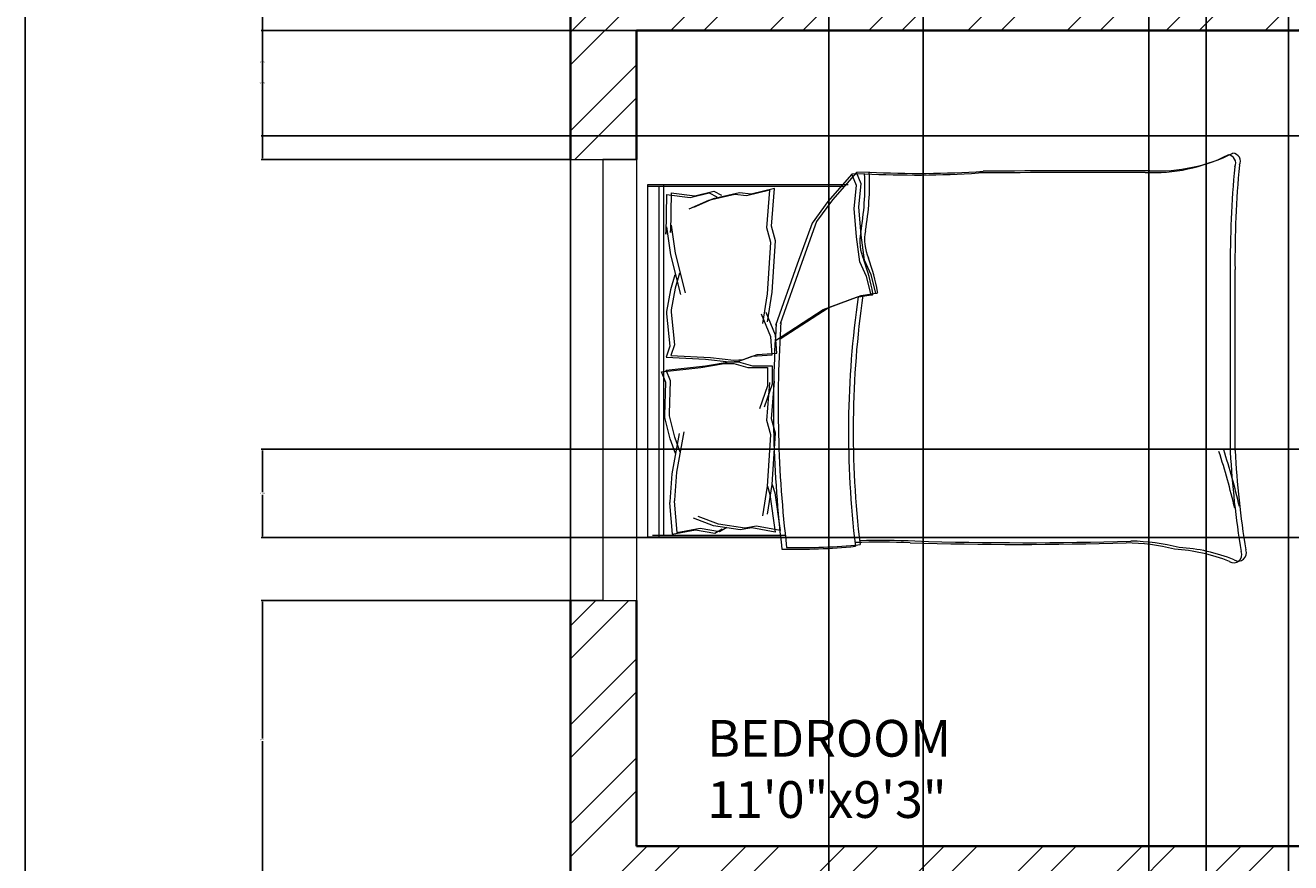
# Model space of a CAD drawing. Units: inches. Extents: x 1748 to 2382, y 1346 to 2284.
# Tile 8 of 26: x 1748 to 1920, y 1857 to 1971. Entities that reach past the tile are written whole.
import ezdxf

# ---------------------------------------------------------------- set-up
doc = ezdxf.new("R2010")
doc.units = ezdxf.units.IN
for name, color, linetype, lineweight in [('A-ANNO-DIMS', 2, 'Continuous', 18), ('A-ANNO-TTLB', 7, 'Continuous', 25), ('A-AREA-IDEN', 7, 'Continuous', 18), ('A-FURN', 8, 'Continuous', 13), ('A-GLAZ', 191, 'Continuous', 18), ('A-WALL', 7, 'Continuous', 35), ('A-WALL-PATT', 9, 'Continuous', 13)]:
    doc.layers.add(name, color=color, linetype=linetype, lineweight=lineweight)
doc.styles.get("Standard").update_dxf_attribs({"font": 'arial.ttf'})
doc.dimstyles.get("Standard").update_dxf_attribs({"dimtxt": 0.18, "dimasz": 0.18, "dimexe": 0.18, "dimexo": 0.0625, "dimgap": 0.09, "dimtad": 0, "dimtih": 1, "dimtoh": 1, "dimdec": 4, "dimzin": 0, "dimdsep": 46, "dimtxsty": 'Standard', "dimcen": 0.09, "dimadec": 0, "dimazin": 0, "dimtfac": 1, "dimtdec": 4, "dimtofl": 0, "dimtmove": 0, "dimatfit": 3, "dimfxl": 1, "dimtolj": 1, "dimtzin": 0, "dimarcsym": 0})

# ---------------------------------------------------------------- blocks, each defined once
blk = doc.blocks.new('BED-DOUBLE')
for p, q in [((3.48, 63.33), (3.48, 81.44)), ((3.48, 63.33), (3.48, 81.44)), ((3.48, 81.44), (51.49, 81.44)), ((51.27, 81.44), (51.27, 54.83)), ((51.27, 81.44), (51.27, 54.83)), ((51.49, 81.44), (51.49, 80.8)), ((3.48, 79.91), (51.27, 79.91)), ((3.48, 79.91), (51.27, 79.91)), ((3.7, 62.69), (3.7, 80.8)), ((3.7, 62.69), (3.7, 80.8)), ((3.7, 79.27), (51.49, 79.27)), ((3.7, 79.27), (51.49, 79.27)), ((24.54, 78.99), (25.98, 79.57)), ((24.54, 78.99), (25.98, 79.57)), ((25.98, 79.57), (26.56, 74.22)), ((25.98, 79.57), (26.56, 74.22)), ((51.49, 80.8), (51.49, 54.19)), ((51.49, 80.8), (51.49, 54.19)), ((3.89, 78.13), (4.47, 74.95)), ((3.9, 78.11), (8.18, 78.43)), ((3.9, 78.11), (8.18, 78.43)), ((3.9, 78.13), (4.47, 74.95)), ((4.12, 77.49), (4.7, 74.31)), ((4.12, 77.49), (4.7, 74.31)), ((4.13, 77.47), (8.41, 77.8)), ((4.13, 77.47), (8.41, 77.8)), ((8.18, 78.43), (8.29, 78.42)), ((8.18, 78.43), (8.28, 78.42)), ((8.28, 78.42), (12.11, 78.13)), ((8.29, 78.42), (12.11, 78.13)), ((8.41, 77.8), (8.51, 77.78)), ((8.41, 77.8), (8.51, 77.78)), ((8.51, 77.78), (12.34, 77.49)), ((8.51, 77.78), (12.34, 77.49)), ((12.11, 78.13), (17.6, 77.12)), ((12.11, 78.13), (17.6, 77.12)), ((12.34, 77.49), (17.83, 76.48)), ((12.34, 77.49), (17.83, 76.48)), ((14.86, 77.69), (16.88, 78.42)), ((14.86, 77.69), (16.88, 78.42)), ((15.08, 77.05), (17.11, 77.78)), ((15.08, 77.05), (17.11, 77.78)), ((16.88, 78.42), (19.77, 79.14)), ((16.88, 78.42), (19.77, 79.14)), ((17.11, 77.78), (20, 78.5)), ((17.11, 77.78), (20, 78.5)), ((19.77, 79.14), (20.09, 79.14)), ((19.77, 79.14), (20.09, 79.14)), ((20, 78.5), (20.32, 78.5)), ((20, 78.5), (20.32, 78.5)), ((20.09, 79.14), (24.54, 78.99)), ((20.09, 79.14), (24.54, 78.99)), ((20.32, 78.5), (24.77, 78.36)), ((20.32, 78.5), (24.77, 78.36)), ((24.77, 78.36), (26.21, 78.93)), ((24.77, 78.36), (26.21, 78.93)), ((26.21, 78.93), (26.79, 73.58)), ((26.21, 78.93), (26.79, 73.58)), ((27.98, 78.95), (27.73, 73.58)), ((27.98, 78.95), (27.73, 73.58)), ((28.21, 78.31), (27.96, 72.94)), ((28.21, 78.31), (27.96, 72.94)), ((29.46, 78.46), (27.98, 78.95)), ((29.46, 78.46), (27.98, 78.95)), ((29.68, 77.83), (28.21, 78.31)), ((29.68, 77.83), (28.21, 78.31)), ((33.88, 78.89), (29.46, 78.46)), ((33.88, 78.89), (29.46, 78.46)), ((34.11, 78.25), (29.68, 77.83)), ((34.11, 78.25), (29.68, 77.83)), ((34.21, 78.91), (33.88, 78.89)), ((34.2, 78.91), (33.88, 78.89)), ((34.43, 78.27), (34.11, 78.25)), ((34.43, 78.27), (34.11, 78.25)), ((37.14, 78.37), (34.2, 78.91)), ((37.14, 78.37), (34.21, 78.91)), ((37.36, 77.73), (34.43, 78.27)), ((37.36, 77.73), (34.43, 78.27)), ((41.91, 78.37), (36.5, 77.02)), ((41.91, 78.37), (36.5, 77.02)), ((42.14, 77.73), (36.72, 76.38)), ((42.14, 77.73), (36.72, 76.38)), ((39.2, 77.77), (37.14, 78.37)), ((39.2, 77.77), (37.14, 78.37)), ((39.43, 77.13), (37.36, 77.73)), ((39.43, 77.13), (37.36, 77.73)), ((45.71, 78.9), (41.91, 78.37)), ((45.71, 78.9), (41.91, 78.37)), ((45.94, 78.26), (42.14, 77.73)), ((45.94, 78.26), (42.14, 77.73)), ((50.11, 78.89), (44.71, 78.98)), ((44.71, 78.98), (45.71, 78.9)), ((50.11, 78.89), (44.71, 78.98)), ((44.71, 78.98), (45.71, 78.9)), ((50.34, 78.25), (44.94, 78.34)), ((44.94, 78.34), (45.94, 78.26)), ((50.34, 78.25), (44.94, 78.34)), ((44.94, 78.34), (45.94, 78.26)), ((50.11, 78.89), (49.73, 75.68)), ((50.11, 78.89), (49.73, 75.68)), ((50.34, 78.25), (49.96, 75.04)), ((50.34, 78.25), (49.96, 75.04)), ((49.31, 73.19), (48.13, 75.87)), ((49.31, 73.19), (48.13, 75.87)), ((4.47, 74.95), (4.04, 72.34)), ((4.47, 74.95), (4.04, 72.34)), ((4.7, 74.31), (4.27, 71.7)), ((4.7, 74.31), (4.27, 71.7)), ((5.05, 72.49), (6.06, 75.24)), ((5.05, 72.49), (6.06, 75.24)), ((5.28, 71.85), (6.29, 74.6)), ((5.28, 71.85), (6.29, 74.6)), ((26.56, 74.22), (27.14, 71.04)), ((26.56, 74.22), (27.14, 71.04)), ((49.54, 72.55), (48.36, 75.23)), ((49.54, 72.55), (48.36, 75.23)), ((49.73, 75.68), (50.33, 73.11)), ((49.73, 75.68), (50.33, 73.11)), ((49.96, 75.04), (50.56, 72.47)), ((49.96, 75.04), (50.56, 72.47)), ((4.04, 72.34), (4.62, 71.33)), ((4.04, 72.34), (4.62, 71.33)), ((4.47, 68.87), (5.05, 72.49)), ((4.47, 68.87), (5.05, 72.49)), ((26.79, 73.58), (27.37, 70.4)), ((26.79, 73.58), (27.37, 70.4)), ((27.73, 73.58), (27.35, 70.37)), ((27.73, 73.58), (27.36, 70.37)), ((27.96, 72.94), (27.58, 69.73)), ((27.96, 72.94), (27.58, 69.73)), ((50.11, 69.61), (49.31, 73.19)), ((50.11, 69.61), (49.31, 73.19)), ((50.34, 68.98), (49.54, 72.55)), ((50.34, 68.98), (49.54, 72.55)), ((50.33, 73.11), (49.81, 72.06)), ((50.33, 73.11), (49.81, 72.06)), ((50.56, 72.47), (50.04, 71.42)), ((50.56, 72.47), (50.04, 71.42)), ((4.27, 71.7), (4.85, 70.69)), ((4.27, 71.7), (4.85, 70.69)), ((4.7, 68.23), (5.28, 71.85)), ((4.7, 68.23), (5.28, 71.85)), ((27.14, 71.04), (27.14, 69.74)), ((27.14, 71.04), (27.14, 69.74)), ((4.76, 67.28), (4.47, 68.87)), ((4.76, 67.28), (4.47, 68.87)), ((27.14, 69.74), (26.56, 67.86)), ((27.14, 69.74), (26.56, 67.86)), ((27.37, 69.1), (26.79, 67.22)), ((27.37, 69.1), (26.79, 67.22)), ((27.35, 70.37), (27.44, 69.07)), ((27.36, 70.37), (27.44, 69.07)), ((27.37, 70.4), (27.37, 69.1)), ((27.37, 70.4), (27.37, 69.1)), ((27.44, 69.07), (28.13, 67.23)), ((27.44, 69.07), (28.13, 67.23)), ((27.58, 69.73), (27.66, 68.43)), ((27.58, 69.73), (27.66, 68.43)), ((49.92, 68.01), (50.11, 69.61)), ((49.92, 68.01), (50.11, 69.61)), ((50.15, 67.37), (50.34, 68.98)), ((50.15, 67.37), (50.34, 68.98)), ((4.18, 64.1), (4.76, 67.28)), ((4.18, 64.1), (4.76, 67.28)), ((4.99, 66.64), (4.7, 68.23)), ((4.99, 66.64), (4.7, 68.23)), ((26.56, 67.86), (26.56, 65.18)), ((26.56, 67.86), (26.56, 65.18)), ((26.79, 67.22), (26.79, 64.54)), ((26.79, 67.22), (26.79, 64.54)), ((27.66, 68.43), (28.36, 66.59)), ((27.66, 68.43), (28.36, 66.59)), ((28.13, 67.23), (28.3, 64.55)), ((28.13, 67.23), (28.3, 64.55)), ((50.7, 64.87), (49.92, 68.01)), ((50.7, 64.87), (49.92, 68.01)), ((50.93, 64.23), (50.15, 67.37)), ((50.93, 64.23), (50.15, 67.37)), ((4.41, 63.46), (4.99, 66.64)), ((4.41, 63.46), (4.99, 66.64)), ((6.38, 65.81), (10.41, 65.15)), ((6.38, 65.81), (10.41, 65.15)), ((24.1, 65.18), (20.96, 66.27)), ((24.1, 65.18), (20.96, 66.27)), ((24.33, 64.54), (21.19, 65.63)), ((24.33, 64.54), (21.19, 65.63)), ((28.36, 66.59), (28.53, 63.91)), ((28.36, 66.59), (28.53, 63.91)), ((30.75, 64.7), (33.82, 65.99)), ((30.75, 64.7), (33.82, 65.99)), ((32.56, 65.81), (36.6, 65.15)), ((32.56, 65.81), (36.6, 65.15)), ((9.28, 64.83), (4.18, 64.1)), ((9.28, 64.83), (4.18, 64.1)), ((9.51, 64.19), (4.41, 63.46)), ((9.51, 64.19), (4.41, 63.46)), ((6.61, 65.18), (10.64, 64.51)), ((6.61, 65.18), (10.64, 64.51)), ((10.41, 65.15), (9.28, 64.83)), ((10.41, 65.15), (9.28, 64.83)), ((10.64, 64.51), (9.51, 64.19)), ((10.64, 64.51), (9.51, 64.19)), ((10.41, 65.15), (17.42, 64.72)), ((10.41, 65.15), (17.42, 64.72)), ((10.64, 64.51), (17.65, 64.08)), ((10.64, 64.51), (17.65, 64.08)), ((17.42, 64.72), (19.38, 65.27)), ((17.42, 64.72), (19.38, 65.27)), ((17.65, 64.08), (19.61, 64.64)), ((17.65, 64.08), (19.61, 64.64)), ((19.38, 65.27), (24.52, 64.87)), ((19.38, 65.27), (24.52, 64.87)), ((19.61, 64.64), (24.74, 64.23)), ((19.61, 64.64), (24.74, 64.23)), ((26.56, 65.18), (24.1, 65.18)), ((26.56, 65.18), (24.1, 65.18)), ((26.79, 64.54), (24.33, 64.54)), ((26.79, 64.54), (24.33, 64.54)), ((28.3, 64.55), (30.75, 64.7)), ((28.3, 64.55), (30.75, 64.7)), ((28.53, 63.91), (30.98, 64.06)), ((28.53, 63.91), (30.98, 64.06)), ((30.26, 64.06), (34.45, 57.57)), ((30.26, 64.06), (34.45, 57.57)), ((30.98, 64.06), (34.05, 65.35)), ((30.98, 64.06), (34.05, 65.35)), ((40.64, 61.13), (32.31, 64.06)), ((40.64, 61.13), (32.31, 64.06)), ((32.79, 65.18), (36.83, 64.51)), ((32.79, 65.18), (36.82, 64.51)), ((36.6, 65.15), (43.61, 64.72)), ((36.6, 65.15), (43.61, 64.72)), ((36.82, 64.51), (43.83, 64.08)), ((36.83, 64.51), (43.83, 64.08)), ((43.61, 64.72), (45.57, 65.27)), ((43.61, 64.72), (45.57, 65.27)), ((43.83, 64.08), (45.8, 64.64)), ((43.83, 64.08), (45.79, 64.64)), ((45.57, 65.27), (50.7, 64.87)), ((45.57, 65.27), (50.7, 64.87)), ((45.79, 64.64), (50.93, 64.23)), ((45.8, 64.64), (50.93, 64.23)), ((30.49, 63.42), (34.68, 56.93)), ((30.49, 63.42), (34.68, 56.93)), ((40.87, 60.49), (32.53, 63.42)), ((40.87, 60.49), (32.53, 63.42)), ((46.22, 59.11), (40.64, 61.13)), ((46.22, 59.11), (40.64, 61.13)), ((46.45, 58.48), (40.87, 60.49)), ((46.45, 58.48), (40.87, 60.49)), ((49.16, 56.95), (46.22, 59.11)), ((49.16, 56.95), (46.22, 59.11)), ((34.45, 57.57), (36.15, 53.08)), ((34.45, 57.57), (36.15, 53.08)), ((34.68, 56.93), (36.38, 52.44)), ((34.68, 56.93), (36.38, 52.44)), ((49.39, 56.31), (46.45, 58.48)), ((49.39, 56.31), (46.45, 58.48)), ((52.87, 53.7), (49.16, 56.95)), ((52.87, 53.7), (49.16, 56.95)), ((53.1, 53.06), (49.39, 56.31)), ((53.1, 53.06), (49.39, 56.31)), ((44.36, 53.08), (48.23, 53.39)), ((44.36, 53.08), (48.23, 53.39)), ((48.23, 53.39), (51.33, 53.08)), ((48.23, 53.39), (51.33, 53.08)), ((51.33, 53.08), (52.87, 53.7)), ((51.33, 53.08), (52.87, 53.7)), ((52.95, 51.95), (52.87, 53.7, 3.87)), ((52.95, 51.95), (52.87, 53.7, 3.87)), ((36.15, 53.08), (36.46, 51.07)), ((36.15, 53.08), (36.46, 51.07)), ((36.38, 52.44), (36.69, 50.43)), ((36.38, 52.44), (36.69, 50.43)), ((36.46, 51.07), (38.94, 51.69)), ((36.46, 51.07), (38.94, 51.69)), ((38.94, 51.69), (40.95, 52.61)), ((38.94, 51.69), (40.95, 52.61)), ((39.17, 51.05), (41.18, 51.97)), ((39.17, 51.05), (41.18, 51.97)), ((40.95, 52.61), (44.36, 53.08)), ((40.95, 52.61), (44.36, 53.08)), ((41.18, 51.97), (44.59, 52.44)), ((41.18, 51.97), (44.59, 52.44)), ((44.59, 52.44), (48.46, 52.75)), ((44.59, 52.44), (48.46, 52.75)), ((48.46, 52.75), (51.56, 52.44)), ((48.46, 52.75), (51.56, 52.44)), ((51.56, 52.44), (53.1, 53.06)), ((51.56, 52.44), (53.1, 53.06)), ((53.18, 51.31), (53.1, 53.06, 3.87)), ((53.18, 51.31), (53.1, 53.06, 3.87)), ((36.69, 50.43), (39.17, 51.05)), ((36.69, 50.43), (39.17, 51.05)), ((15.06, 2.2), (39.68, 2.2)), ((15.06, 2.2), (39.68, 2.2)), ((15.29, 1.56), (39.91, 1.56)), ((15.29, 1.56), (39.91, 1.56))]:
    blk.add_line(p, q)
for centre, radius, start, end in [((21.36, -100.61), 164.97, 86.0865, 96.7821), ((21.36, -100.61), 164.97, 86.0865, 96.7821), ((21.59, -101.25), 164.97, 86.0865, 96.7821), ((21.59, -101.25), 164.97, 86.0865, 96.7821), ((85.16, 61.35), 83.31, 178.7218, 185.604), ((85.16, 61.35), 83.31, 178.7218, 185.604), ((85.39, 60.71), 83.31, 178.7218, 185.604), ((85.39, 60.71), 83.31, 178.7218, 185.604), ((17.76, -74.87), 129.02, 81.7845, 96.9006), ((17.76, -74.87), 129.02, 81.7845, 96.9006), ((17.98, -75.51), 129.02, 81.7845, 96.9006), ((17.98, -75.51), 129.02, 81.7845, 96.9006), ((-167.31, 50.27), 170.11, 358.4762, 1.0082), ((-167.31, 50.27), 170.11, 358.4762, 1.0082), ((-167.08, 49.63), 170.11, 358.4762, 1.0082), ((-167.08, 49.63), 170.11, 358.4762, 1.0082), ((31.15, 79.96), 29.65, 280.6617, 289.8806), ((31.15, 79.96), 29.65, 280.6617, 289.8806), ((43.74, 46.38), 6.22, 78.6608, 113.7384), ((43.74, 46.38), 6.22, 78.6608, 113.7384), ((43.97, 45.74), 6.22, 78.6608, 113.7384), ((43.97, 45.74), 6.22, 78.6608, 113.7384), ((51.33, 88.1), 36.18, 259.8763, 272.5657), ((51.33, 88.1), 36.18, 259.8763, 272.5657), ((51.56, 87.46), 36.18, 259.8763, 272.5657), ((51.56, 87.46), 36.18, 259.8763, 272.5657), ((182.27, 45.13), 129.5, 176.9791, 183.8365), ((182.27, 45.13), 129.5, 176.9791, 183.8365), ((36.64, 51), 0.185, 160.2464, 271.1377), ((36.64, 51), 0.185, 160.2464, 271.1377), ((36.87, 50.36), 0.185, 160.2464, 271.1377), ((36.86, 50.36), 0.185, 160.2464, 271.1377), ((31.38, 79.32), 29.65, 280.6617, 289.8806), ((31.38, 79.32), 29.65, 280.6617, 289.8806), ((182.49, 44.49), 129.5, 176.9791, 183.8365), ((182.49, 44.49), 129.5, 176.9791, 183.8365), ((484.82, 30.83), 482.31, 178.2277, 181.7185), ((484.82, 30.83), 482.31, 178.2277, 181.7185), ((485.05, 30.19), 482.31, 178.2277, 181.7185), ((485.05, 30.19), 482.31, 178.2277, 181.7185), ((-4508.74, 13.62), 4561.86, 0.00217, 0.28689), ((-4508.74, 13.62), 4561.86, 0.00217, 0.28689), ((-4508.51, 12.98), 4561.86, 0.00217, 0.28689), ((-4508.51, 12.98), 4561.86, 0.00217, 0.28689), ((-26.9, 16.93), 29.63, 346.0648, 358.9113), ((-26.9, 16.93), 29.63, 346.0648, 358.9113), ((-26.67, 16.29), 29.63, 346.0648, 358.9113), ((-26.67, 16.29), 29.63, 346.0648, 358.9113), ((76.16, 12.78), 23.07, 177.4714, 206.4681), ((76.16, 12.78), 23.07, 177.4714, 206.4681), ((76.39, 12.14), 23.07, 177.4714, 206.4681), ((76.39, 12.14), 23.07, 177.4714, 206.4681), ((-21.66, 11.17), 23.56, 337.9751, 356.652), ((-21.66, 11.17), 23.56, 337.9751, 356.652), ((-21.43, 10.53), 23.56, 337.9751, 356.652), ((-21.43, 10.53), 23.56, 337.9751, 356.652), ((-17.22, 105.16), 106.46, 283.3832, 287.7053), ((-17.22, 105.16), 106.46, 283.3832, 287.7053), ((1.09, 1.73), 1.09, 146.1736, 293.4781), ((1.09, 1.73), 1.09, 146.1736, 293.4781), ((21.43, -119.39), 121.76, 92.9958, 99.4091), ((21.43, -119.39), 121.76, 92.9958, 99.4091), ((-16.99, 104.52), 106.46, 283.3832, 287.7053), ((-16.99, 104.52), 106.46, 283.3832, 287.7053), ((41.15, -130.83), 133.04, 84.4998, 90.6351), ((41.15, -130.83), 133.04, 84.4998, 90.6351), ((54.41, 2.57), 1.1, 242.6588, 356.02), ((54.41, 2.57), 1.1, 242.6588, 356.02), ((54.64, 1.93), 1.1, 242.6588, 356.02), ((54.64, 1.93), 1.1, 242.6588, 356.02), ((1.32, 1.09), 1.09, 146.1736, 293.4781), ((1.32, 1.09), 1.09, 146.1736, 293.4781), ((21.66, -120.03), 121.76, 92.9958, 99.4091), ((21.66, -120.03), 121.76, 92.9958, 99.4091), ((41.38, -131.47), 133.04, 84.4998, 90.6351), ((41.38, -131.47), 133.04, 84.4998, 90.6351)]:
    blk.add_arc(centre, radius, start, end)
blk = doc.blocks.new('*D37')
at = {"layer": 'A-ANNO-DIMS', "color": 0, "lineweight": -2, "transparency": 16777216}
for p, q in [((2031.9, 1970.35), (1779.88, 1970.35)), ((1780.06, 1970.17), (1780.06, 1963.37)), ((1780.06, 1956.2), (1780.06, 1963.01)), ((2031.9, 1956.02), (1779.88, 1956.02))]:
    blk.add_line(p, q, dxfattribs=at)
at = {"layer": 'A-ANNO-DIMS', "color": 0, "transparency": 16777216}
for points in [[(1780.03, 1970.17), (1780.09, 1970.17), (1780.06, 1970.35)], [(1780.03, 1956.2), (1780.09, 1956.2), (1780.06, 1956.02)]]:
    blk.add_solid(points, dxfattribs=at)
at = {"layer": 'Defpoints', "color": 0, "transparency": 16777216}
for p in [(1780.06, 1970.35), (2031.96, 1970.35), (2031.96, 1956.02)]:
    blk.add_point(p, dxfattribs=at)
at = {"layer": 'A-ANNO-DIMS', "color": 0, "transparency": 16777216, "insert": (1780.06, 1963.19), "char_height": 0.18, "attachment_point": 5}
blk.add_mtext('\\A1;14.325', dxfattribs=at)
blk = doc.blocks.new('*D41')
at = {"layer": 'A-ANNO-DIMS', "color": 0, "lineweight": -2, "transparency": 16777216}
for p, q in [((1821.96, 1854.91), (1821.96, 2274.93)), ((1822.14, 2274.75), (1839.16, 2274.75)), ((1856.96, 2274.75), (1839.95, 2274.75)), ((1857.14, 1854.91), (1857.14, 2274.93))]:
    blk.add_line(p, q, dxfattribs=at)
at = {"layer": 'A-ANNO-DIMS', "color": 0, "transparency": 16777216}
for points in [[(1822.14, 2274.78), (1822.14, 2274.72), (1821.96, 2274.75)], [(1856.96, 2274.78), (1856.96, 2274.72), (1857.14, 2274.75)]]:
    blk.add_solid(points, dxfattribs=at)
at = {"layer": 'Defpoints', "color": 0, "transparency": 16777216}
for p in [(1857.14, 2274.75), (1821.96, 1854.85), (1857.14, 1854.85)]:
    blk.add_point(p, dxfattribs=at)
at = {"layer": 'A-ANNO-DIMS', "color": 0, "transparency": 16777216, "insert": (1839.55, 2274.75), "char_height": 0.18, "attachment_point": 5}
blk.add_mtext('\\A1;35.18', dxfattribs=at)
blk = doc.blocks.new('*D44')
at = {"layer": 'A-ANNO-DIMS', "color": 0, "lineweight": -2, "transparency": 16777216}
for p, q in [((1821.9, 1892.79), (1779.88, 1892.79)), ((1780.06, 1892.61), (1780.06, 1874)), ((1780.06, 1855.03), (1780.06, 1873.64)), ((1821.9, 1854.85), (1779.88, 1854.85))]:
    blk.add_line(p, q, dxfattribs=at)
at = {"layer": 'A-ANNO-DIMS', "color": 0, "transparency": 16777216}
for points in [[(1780.03, 1892.61), (1780.09, 1892.61), (1780.06, 1892.79)], [(1780.03, 1855.03), (1780.09, 1855.03), (1780.06, 1854.85)]]:
    blk.add_solid(points, dxfattribs=at)
at = {"layer": 'Defpoints', "color": 0, "transparency": 16777216}
for p in [(1780.06, 1892.79), (1821.96, 1892.79), (1821.96, 1854.85)]:
    blk.add_point(p, dxfattribs=at)
at = {"layer": 'A-ANNO-DIMS', "color": 0, "transparency": 16777216, "insert": (1780.06, 1873.82), "char_height": 0.18, "attachment_point": 5}
blk.add_mtext('\\A1;37.94', dxfattribs=at)
blk = doc.blocks.new('*D50')
at = {"layer": 'A-ANNO-DIMS', "color": 0, "lineweight": -2, "transparency": 16777216}
for p, q in [((1869.96, 2223.79), (1869.96, 1360.47)), ((1908.44, 2223.79), (1908.44, 1360.47)), ((1870.14, 1360.65), (1888.81, 1360.65)), ((1908.26, 1360.65), (1889.6, 1360.65))]:
    blk.add_line(p, q, dxfattribs=at)
at = {"layer": 'A-ANNO-DIMS', "color": 0, "transparency": 16777216}
for points in [[(1870.14, 1360.68), (1870.14, 1360.62), (1869.96, 1360.65)], [(1908.26, 1360.68), (1908.26, 1360.62), (1908.44, 1360.65)]]:
    blk.add_solid(points, dxfattribs=at)
at = {"layer": 'Defpoints', "color": 0, "transparency": 16777216}
for p in [(1869.96, 2223.85), (1908.44, 2223.85), (1908.44, 1360.65)]:
    blk.add_point(p, dxfattribs=at)
at = {"layer": 'A-ANNO-DIMS', "color": 0, "transparency": 16777216, "insert": (1889.2, 1360.65), "char_height": 0.18, "attachment_point": 5}
blk.add_mtext('\\A1;38.48', dxfattribs=at)
blk = doc.blocks.new('*D56')
at = {"layer": 'A-ANNO-DIMS', "color": 0, "lineweight": -2, "transparency": 16777216}
for p, q in [((2288.4, 1913.35), (1779.88, 1913.35)), ((1780.06, 1913.17), (1780.06, 1907.52)), ((1780.06, 1901.51), (1780.06, 1907.16)), ((2288.4, 1901.33), (1779.88, 1901.33))]:
    blk.add_line(p, q, dxfattribs=at)
at = {"layer": 'A-ANNO-DIMS', "color": 0, "transparency": 16777216}
for points in [[(1780.03, 1913.17), (1780.09, 1913.17), (1780.06, 1913.35)], [(1780.03, 1901.51), (1780.09, 1901.51), (1780.06, 1901.33)]]:
    blk.add_solid(points, dxfattribs=at)
at = {"layer": 'Defpoints', "color": 0, "transparency": 16777216}
for p in [(1780.06, 1913.35), (2288.46, 1913.35), (2288.46, 1901.33)]:
    blk.add_point(p, dxfattribs=at)
at = {"layer": 'A-ANNO-DIMS', "color": 0, "transparency": 16777216, "insert": (1780.06, 1907.34), "char_height": 0.18, "attachment_point": 5}
blk.add_mtext('\\A1;12.023', dxfattribs=at)
blk = doc.blocks.new('*D64')
at = {"layer": 'A-ANNO-DIMS', "color": 0, "lineweight": -2, "transparency": 16777216}
for p, q in [((1900.64, 1476.91), (1900.64, 2274.93)), ((1900.82, 2274.75), (1909.7, 2274.75)), ((1919.5, 2274.75), (1910.62, 2274.75)), ((1919.68, 1476.91), (1919.68, 2274.93))]:
    blk.add_line(p, q, dxfattribs=at)
at = {"layer": 'A-ANNO-DIMS', "color": 0, "transparency": 16777216}
for points in [[(1900.82, 2274.78), (1900.82, 2274.72), (1900.64, 2274.75)], [(1919.5, 2274.78), (1919.5, 2274.72), (1919.68, 2274.75)]]:
    blk.add_solid(points, dxfattribs=at)
at = {"layer": 'Defpoints', "color": 0, "transparency": 16777216}
for p in [(1919.68, 2274.75), (1900.64, 1476.85), (1919.68, 1476.85)]:
    blk.add_point(p, dxfattribs=at)
at = {"layer": 'A-ANNO-DIMS', "color": 0, "transparency": 16777216, "insert": (1910.16, 2274.75), "char_height": 0.18, "attachment_point": 5}
blk.add_mtext('\\A1;19.035', dxfattribs=at)
blk = doc.blocks.new('*D72')
at = {"layer": 'A-ANNO-DIMS', "color": 0, "lineweight": -2, "transparency": 16777216}
for p, q in [((1821.9, 1979.35), (1779.88, 1979.35)), ((1780.06, 1979.17), (1780.06, 1966.25)), ((1780.06, 1952.97), (1780.06, 1965.89)), ((1821.9, 1952.79), (1779.88, 1952.79))]:
    blk.add_line(p, q, dxfattribs=at)
at = {"layer": 'A-ANNO-DIMS', "color": 0, "transparency": 16777216}
for points in [[(1780.03, 1979.17), (1780.09, 1979.17), (1780.06, 1979.35)], [(1780.03, 1952.97), (1780.09, 1952.97), (1780.06, 1952.79)]]:
    blk.add_solid(points, dxfattribs=at)
at = {"layer": 'Defpoints', "color": 0, "transparency": 16777216}
for p in [(1780.06, 1979.35), (1821.96, 1979.35), (1821.96, 1952.79)]:
    blk.add_point(p, dxfattribs=at)
at = {"layer": 'A-ANNO-DIMS', "color": 0, "transparency": 16777216, "insert": (1780.06, 1966.07), "char_height": 0.18, "attachment_point": 5}
blk.add_mtext('\\A1;26.56', dxfattribs=at)

msp = doc.modelspace()

# ---------------------------------------------------------------- hatches: boundary and pattern name
at = {"layer": 'A-WALL-PATT'}
h = msp.add_hatch(dxfattribs=at)
h.set_pattern_fill('ANSI32', color=256)
h.paths.add_polyline_path([(1908.4445, 2232.8497), (1821.9607, 2232.8497), (1821.9607, 2223.8497), (1865.4607, 2223.8497), (1865.4607, 2209.9185), (1869.9607, 2209.9185), (1869.9607, 2223.8497), (1908.4445, 2223.8497), (1908.4445, 2228.3497)])
h.paths.add_polyline_path([(2040.0683, 2232.8497), (1968.4445, 2232.8497), (1968.4445, 2223.8497), (2025.9607, 2223.8497), (2025.9607, 2130.3497), (2032.1341, 2130.3497), (2032.1341, 2132.5997), (2032.1341, 2134.8497), (2030.4607, 2134.8497), (2030.4607, 2223.8497), (2040.0683, 2223.8497)])
h.paths.add_polyline_path([(2091.3969, 2232.8497), (2064.0683, 2232.8497), (2064.0683, 2223.8497), (2078.4607, 2223.8497), (2078.4607, 2134.8497), (2051.1563, 2134.8497), (2051.1563, 2130.3497), (2078.4607, 2130.3497), (2078.4607, 2128.6813), (2082.9607, 2128.6813), (2082.9607, 2130.3497), (2086.1879, 2130.3497), (2086.1879, 2132.5997), (2086.1879, 2134.8497), (2082.9607, 2134.8497), (2082.9607, 2223.8497), (2091.3969, 2223.8497), (2091.3969, 2228.3497)])
h.paths.add_polyline_path([(2167.0164, 2232.8497), (2115.3969, 2232.8497), (2115.3969, 2223.8497), (2130.9607, 2223.8497), (2130.9607, 2134.8497), (2106.9607, 2134.8497), (2106.9607, 2130.3497), (2135.4607, 2130.3497), (2135.4607, 2223.8497), (2167.0164, 2223.8497), (2167.0164, 2228.3497)])
h.paths.add_polyline_path([(1869.9607, 2149.9185), (1865.4607, 2149.9185), (1865.4607, 2127.8942), (1869.9607, 2127.8942)])
h.paths.add_polyline_path([(2082.9607, 2104.4871), (2080.7107, 2104.4871), (2078.4607, 2104.4871), (2078.4607, 2103.8497), (1869.9607, 2103.8497), (1869.9607, 2108.6062), (1867.7107, 2108.6062), (1865.4607, 2108.6062), (1865.4607, 2103.8497), (1821.9607, 2103.8497), (1821.9607, 2099.3497), (1865.4607, 2099.3497), (1865.4607, 2094.7509), (1869.9607, 2094.7509), (1869.9607, 2099.3497), (2025.9607, 2099.3497), (2025.9607, 2096.4326), (2030.4607, 2096.4326), (2030.4607, 2099.3497), (2082.9607, 2099.3497)])
h.paths.add_polyline_path([(1928.9457, 1401.1212), (2176.8693, 1401.1212), (2176.8693, 1438.214), (1928.9457, 1438.214)], flags=9)
h.paths.add_polyline_path([(2122.2668, 2048.1927), (2177.9387, 2048.1927), (2177.9387, 2066.85), (2122.2668, 2066.85)], flags=9)
h.paths.add_polyline_path([(2272.688, 2153.8197), (2272.688, 2216.746), (2262.3845, 2216.746), (2262.3845, 2153.8197)], flags=9)
h.paths.add_polyline_path([(2157.2928, 2166.5593), (2196.3822, 2166.5593), (2196.3822, 2185.2167), (2157.2928, 2185.2167)], flags=9)
h.paths.add_polyline_path([(2089.3407, 2162.0698), (2124.3987, 2162.0698), (2124.3987, 2180.7272), (2089.3407, 2180.7272)], flags=9)
h.paths.add_polyline_path([(2037.4521, 2160.0913), (2072.5101, 2160.0913), (2072.5101, 2178.7486), (2037.4521, 2178.7486)], flags=9)
h.paths.add_polyline_path([(1884.7894, 2104.1554), (1923.6297, 2104.1554), (1923.6297, 2122.8127), (1884.7894, 2122.8127)], flags=9)
h.paths.add_polyline_path([(1851.2832, 2142.9749), (1851.2832, 2199.3051), (1840.9796, 2199.3051), (1840.9796, 2142.9749)], flags=9)
h.paths.add_polyline_path([(1844.8763, 2017.2834), (1844.8763, 2073.6136), (1834.5728, 2073.6136), (1834.5728, 2017.2834)], flags=9)
h.paths.add_polyline_path([(1897.1577, 2073.1279), (1935.9981, 2073.1279), (1935.9981, 2091.7853), (1897.1577, 2091.7853)], flags=9)
h.paths.add_polyline_path([(1952.3395, 1802.4231), (2008.0114, 1802.4231), (2008.0114, 1821.0805), (1952.3395, 1821.0805)], flags=9)
h.paths.add_polyline_path([(1978.8184, 1857.6841), (2017.7338, 1857.6841), (2017.7338, 1876.3415), (1978.8184, 1876.3415)], flags=9)
h.paths.add_polyline_path([(1979.6513, 1925.9516), (2008.8089, 1925.9516), (2008.8089, 1944.6089), (1979.6513, 1944.6089)], flags=9)
h.paths.add_polyline_path([(1838.5553, 1860.3527), (1877.3957, 1860.3527), (1877.3957, 1879.01), (1838.5553, 1879.01)], flags=9)
h.paths.add_polyline_path([(1883.9018, 1787.3013), (1883.9018, 1843.6315), (1873.5983, 1843.6315), (1873.5983, 1787.3013)], flags=9)
h.paths.add_polyline_path([(1873.7079, 1509.1938), (1873.7079, 1583.7709), (1863.4044, 1583.7709), (1863.4044, 1509.1938)], flags=9)
h.paths.add_polyline_path([(1916.2259, 1603.3681), (1955.0663, 1603.3681), (1955.0663, 1622.0254), (1916.2259, 1622.0254)], flags=9)
h.paths.add_polyline_path([(1876.3013, 1636.757), (1876.3013, 1693.0871), (1865.9978, 1693.0871), (1865.9978, 1636.757)], flags=9)
h.paths.add_polyline_path([(1921.3138, 1521.8316), (1964.0662, 1521.8316), (1964.0662, 1540.489), (1921.3138, 1540.489)], flags=9)
h.paths.add_polyline_path([(2017.5657, 1497.5078), (2046.7983, 1497.5078), (2046.7983, 1516.1651), (2017.5657, 1516.1651)], flags=9)
h.paths.add_polyline_path([(2066.8661, 1499.3902), (2096.0988, 1499.3902), (2096.0988, 1518.0475), (2066.8661, 1518.0475)], flags=9)
h.paths.add_polyline_path([(2155.4835, 1571.6596), (2198.2358, 1571.6596), (2198.2358, 1590.3169), (2155.4835, 1590.3169)], flags=9)
h.paths.add_polyline_path([(2094.9136, 1664.6812), (2150.5855, 1664.6812), (2150.5855, 1683.3386), (2094.9136, 1683.3386)], flags=9)
h.paths.add_polyline_path([(2257.6902, 1863.1628), (2269.8935, 1863.1628), (2269.8935, 1873.4664), (2257.6902, 1873.4664)], flags=9)
h.paths.add_polyline_path([(2164.0748, 1880.3089), (2189.8694, 1880.3089), (2189.8694, 1890.6124), (2164.0748, 1890.6124)], flags=9)
h.paths.add_polyline_path([(2239.4394, 1931.0585), (2268.8187, 1931.0585), (2268.8187, 1949.7159), (2239.4394, 1949.7159)], flags=9)
h = msp.add_hatch(dxfattribs=at)
h.set_pattern_fill('ANSI32', color=256)
h.paths.add_polyline_path([(2297.4607, 2232.8497), (2203.0164, 2232.8497), (2203.0164, 2223.8497), (2244.9607, 2223.8497), (2244.9607, 2127.8554), (2249.4607, 2127.8554), (2249.4607, 2223.8497), (2297.4607, 2223.8497)])
h.paths.add_polyline_path([(2297.4607, 2103.8497), (2249.4607, 2103.8497), (2249.4607, 2106.7497), (2247.2107, 2106.7497), (2244.9607, 2106.7497), (2244.9607, 2103.8497), (2130.9607, 2103.8497), (2130.9607, 2099.3497), (2288.4607, 2099.3497), (2288.4607, 2077.2008), (2297.4607, 2077.2008)])
h.paths.add_polyline_path([(1928.9457, 1401.1212), (2176.8693, 1401.1212), (2176.8693, 1438.214), (1928.9457, 1438.214)], flags=9)
h.paths.add_polyline_path([(2122.2668, 2048.1927), (2177.9387, 2048.1927), (2177.9387, 2066.85), (2122.2668, 2066.85)], flags=9)
h.paths.add_polyline_path([(2272.688, 2153.8197), (2272.688, 2216.746), (2262.3845, 2216.746), (2262.3845, 2153.8197)], flags=25)
h.paths.add_polyline_path([(2157.2928, 2166.5593), (2196.3822, 2166.5593), (2196.3822, 2185.2167), (2157.2928, 2185.2167)], flags=9)
h.paths.add_polyline_path([(2089.3407, 2162.0698), (2124.3987, 2162.0698), (2124.3987, 2180.7272), (2089.3407, 2180.7272)], flags=9)
h.paths.add_polyline_path([(2037.4521, 2160.0913), (2072.5101, 2160.0913), (2072.5101, 2178.7486), (2037.4521, 2178.7486)], flags=9)
h.paths.add_polyline_path([(1884.7894, 2104.1554), (1923.6297, 2104.1554), (1923.6297, 2122.8127), (1884.7894, 2122.8127)], flags=9)
h.paths.add_polyline_path([(1851.2832, 2142.9749), (1851.2832, 2199.3051), (1840.9796, 2199.3051), (1840.9796, 2142.9749)], flags=9)
h.paths.add_polyline_path([(1844.8763, 2017.2834), (1844.8763, 2073.6136), (1834.5728, 2073.6136), (1834.5728, 2017.2834)], flags=9)
h.paths.add_polyline_path([(1897.1577, 2073.1279), (1935.9981, 2073.1279), (1935.9981, 2091.7853), (1897.1577, 2091.7853)], flags=9)
h.paths.add_polyline_path([(1952.3395, 1802.4231), (2008.0114, 1802.4231), (2008.0114, 1821.0805), (1952.3395, 1821.0805)], flags=9)
h.paths.add_polyline_path([(1978.8184, 1857.6841), (2017.7338, 1857.6841), (2017.7338, 1876.3415), (1978.8184, 1876.3415)], flags=9)
h.paths.add_polyline_path([(1979.6513, 1925.9516), (2008.8089, 1925.9516), (2008.8089, 1944.6089), (1979.6513, 1944.6089)], flags=9)
h.paths.add_polyline_path([(1838.5553, 1860.3527), (1877.3957, 1860.3527), (1877.3957, 1879.01), (1838.5553, 1879.01)], flags=9)
h.paths.add_polyline_path([(1883.9018, 1787.3013), (1883.9018, 1843.6315), (1873.5983, 1843.6315), (1873.5983, 1787.3013)], flags=9)
h.paths.add_polyline_path([(1873.7079, 1509.1938), (1873.7079, 1583.7709), (1863.4044, 1583.7709), (1863.4044, 1509.1938)], flags=9)
h.paths.add_polyline_path([(1916.2259, 1603.3681), (1955.0663, 1603.3681), (1955.0663, 1622.0254), (1916.2259, 1622.0254)], flags=9)
h.paths.add_polyline_path([(1876.3013, 1636.757), (1876.3013, 1693.0871), (1865.9978, 1693.0871), (1865.9978, 1636.757)], flags=9)
h.paths.add_polyline_path([(1921.3138, 1521.8316), (1964.0662, 1521.8316), (1964.0662, 1540.489), (1921.3138, 1540.489)], flags=9)
h.paths.add_polyline_path([(2017.5657, 1497.5078), (2046.7983, 1497.5078), (2046.7983, 1516.1651), (2017.5657, 1516.1651)], flags=9)
h.paths.add_polyline_path([(2066.8661, 1499.3902), (2096.0988, 1499.3902), (2096.0988, 1518.0475), (2066.8661, 1518.0475)], flags=9)
h.paths.add_polyline_path([(2155.4835, 1571.6596), (2198.2358, 1571.6596), (2198.2358, 1590.3169), (2155.4835, 1590.3169)], flags=9)
h.paths.add_polyline_path([(2094.9136, 1664.6812), (2150.5855, 1664.6812), (2150.5855, 1683.3386), (2094.9136, 1683.3386)], flags=9)
h.paths.add_polyline_path([(2257.6902, 1863.1628), (2269.8935, 1863.1628), (2269.8935, 1873.4664), (2257.6902, 1873.4664)], flags=9)
h.paths.add_polyline_path([(2164.0748, 1880.3089), (2189.8694, 1880.3089), (2189.8694, 1890.6124), (2164.0748, 1890.6124)], flags=9)
h.paths.add_polyline_path([(2239.4394, 1931.0585), (2268.8187, 1931.0585), (2268.8187, 1949.7159), (2239.4394, 1949.7159)], flags=9)
h = msp.add_hatch(dxfattribs=at)
h.set_pattern_fill('ANSI32', color=256)
h.paths.add_polyline_path([(1919.6777, 1476.8497), (1900.6426, 1476.8497), (1900.6426, 1522.0826), (1898.3926, 1522.0826), (1896.1426, 1522.0826), (1896.1426, 1476.8497), (1857.1426, 1476.8497), (1857.1426, 1467.8497), (1896.1426, 1467.8497), (1919.6777, 1467.8497), (1919.6777, 1472.3497)])
h.paths.add_polyline_path([(2018.7873, 1472.3497), (2018.7873, 1476.8497), (2010.9607, 1476.8497), (2010.9607, 1560.8497), (2034.9607, 1560.8497), (2034.9607, 1565.3497), (2006.4607, 1565.3497), (2006.4607, 1476.8497), (1955.6777, 1476.8497), (1955.6777, 1467.8497), (2018.7873, 1467.8497)])
h.paths.add_polyline_path([(2152.3354, 1472.3497), (2152.3354, 1476.8497), (2115.9607, 1476.8497), (2115.9607, 1565.3497), (2109.2204, 1565.3497), (2109.2204, 1563.0997), (2109.2204, 1560.8497), (2111.4607, 1560.8497), (2111.4607, 1476.8497), (2095.3617, 1476.8497), (2095.3617, 1467.8497), (2152.3354, 1467.8497)])
h.paths.add_polyline_path([(2071.3617, 1476.8497), (2063.4607, 1476.8497), (2063.4607, 1560.8497), (2090.1865, 1560.8497), (2090.1865, 1565.3497), (2063.4607, 1565.3497), (2063.4607, 1572.5485), (2061.2107, 1572.5485), (2058.9607, 1572.5485), (2058.9607, 1565.3497), (2055.6281, 1565.3497), (2055.6281, 1560.8497), (2058.9607, 1560.8497), (2058.9607, 1476.8497), (2042.7873, 1476.8497), (2042.7873, 1467.8497), (2071.3617, 1467.8497), (2071.3617, 1472.3497)])
h.paths.add_polyline_path([(2297.4607, 1506.5652), (2288.4607, 1506.5652), (2288.4607, 1476.8497), (2212.3354, 1476.8497), (2212.3354, 1467.8497), (2297.4607, 1467.8497)])
h.paths.add_polyline_path([(2297.4607, 1645.3038), (2288.4607, 1645.3038), (2288.4607, 1605.8497), (2058.9607, 1605.8497), (2058.9607, 1600.1857), (2061.2107, 1600.1857), (2063.4607, 1600.1857), (2063.4607, 1601.3497), (2288.4607, 1601.3497), (2288.4607, 1566.5652), (2297.4607, 1566.5652)])
h.paths.add_polyline_path([(2010.9607, 1609.0561), (2008.7107, 1609.0561), (2006.4607, 1609.0561), (2006.4607, 1605.8497), (1900.6426, 1605.8497), (1900.6426, 1609.7171), (1898.3926, 1609.7171), (1896.1426, 1609.7171), (1896.1426, 1605.8497), (1857.1426, 1605.8497), (1857.1426, 1601.3497), (1896.1426, 1601.3497), (1896.1426, 1542.5447), (1900.6426, 1542.5447), (1900.6426, 1601.3497), (2010.9607, 1601.3497)])
h.paths.add_polyline_path([(1928.9457, 1401.1212), (2176.8693, 1401.1212), (2176.8693, 1438.214), (1928.9457, 1438.214)], flags=9)
h.paths.add_polyline_path([(2122.2668, 2048.1927), (2177.9387, 2048.1927), (2177.9387, 2066.85), (2122.2668, 2066.85)], flags=9)
h.paths.add_polyline_path([(2272.688, 2153.8197), (2272.688, 2216.746), (2262.3845, 2216.746), (2262.3845, 2153.8197)], flags=9)
h.paths.add_polyline_path([(2157.2928, 2166.5593), (2196.3822, 2166.5593), (2196.3822, 2185.2167), (2157.2928, 2185.2167)], flags=9)
h.paths.add_polyline_path([(2089.3407, 2162.0698), (2124.3987, 2162.0698), (2124.3987, 2180.7272), (2089.3407, 2180.7272)], flags=9)
h.paths.add_polyline_path([(2037.4521, 2160.0913), (2072.5101, 2160.0913), (2072.5101, 2178.7486), (2037.4521, 2178.7486)], flags=9)
h.paths.add_polyline_path([(1884.7894, 2104.1554), (1923.6297, 2104.1554), (1923.6297, 2122.8127), (1884.7894, 2122.8127)], flags=9)
h.paths.add_polyline_path([(1851.2832, 2142.9749), (1851.2832, 2199.3051), (1840.9796, 2199.3051), (1840.9796, 2142.9749)], flags=9)
h.paths.add_polyline_path([(1844.8763, 2017.2834), (1844.8763, 2073.6136), (1834.5728, 2073.6136), (1834.5728, 2017.2834)], flags=9)
h.paths.add_polyline_path([(1897.1577, 2073.1279), (1935.9981, 2073.1279), (1935.9981, 2091.7853), (1897.1577, 2091.7853)], flags=9)
h.paths.add_polyline_path([(1952.3395, 1802.4231), (2008.0114, 1802.4231), (2008.0114, 1821.0805), (1952.3395, 1821.0805)], flags=9)
h.paths.add_polyline_path([(1978.8184, 1857.6841), (2017.7338, 1857.6841), (2017.7338, 1876.3415), (1978.8184, 1876.3415)], flags=9)
h.paths.add_polyline_path([(1979.6513, 1925.9516), (2008.8089, 1925.9516), (2008.8089, 1944.6089), (1979.6513, 1944.6089)], flags=9)
h.paths.add_polyline_path([(1838.5553, 1860.3527), (1877.3957, 1860.3527), (1877.3957, 1879.01), (1838.5553, 1879.01)], flags=9)
h.paths.add_polyline_path([(1883.9018, 1787.3013), (1883.9018, 1843.6315), (1873.5983, 1843.6315), (1873.5983, 1787.3013)], flags=9)
h.paths.add_polyline_path([(1873.7079, 1509.1938), (1873.7079, 1583.7709), (1863.4044, 1583.7709), (1863.4044, 1509.1938)], flags=9)
h.paths.add_polyline_path([(1916.2259, 1603.3681), (1955.0663, 1603.3681), (1955.0663, 1622.0254), (1916.2259, 1622.0254)], flags=9)
h.paths.add_polyline_path([(1876.3013, 1636.757), (1876.3013, 1693.0871), (1865.9978, 1693.0871), (1865.9978, 1636.757)], flags=9)
h.paths.add_polyline_path([(1921.3138, 1521.8316), (1964.0662, 1521.8316), (1964.0662, 1540.489), (1921.3138, 1540.489)], flags=9)
h.paths.add_polyline_path([(2017.5657, 1497.5078), (2046.7983, 1497.5078), (2046.7983, 1516.1651), (2017.5657, 1516.1651)], flags=9)
h.paths.add_polyline_path([(2066.8661, 1499.3902), (2096.0988, 1499.3902), (2096.0988, 1518.0475), (2066.8661, 1518.0475)], flags=9)
h.paths.add_polyline_path([(2155.4835, 1571.6596), (2198.2358, 1571.6596), (2198.2358, 1590.3169), (2155.4835, 1590.3169)], flags=25)
h.paths.add_polyline_path([(2094.9136, 1664.6812), (2150.5855, 1664.6812), (2150.5855, 1683.3386), (2094.9136, 1683.3386)], flags=9)
h.paths.add_polyline_path([(2257.6902, 1863.1628), (2269.8935, 1863.1628), (2269.8935, 1873.4664), (2257.6902, 1873.4664)], flags=9)
h.paths.add_polyline_path([(2164.0748, 1880.3089), (2189.8694, 1880.3089), (2189.8694, 1890.6124), (2164.0748, 1890.6124)], flags=9)
h.paths.add_polyline_path([(2239.4394, 1931.0585), (2268.8187, 1931.0585), (2268.8187, 1949.7159), (2239.4394, 1949.7159)], flags=9)
h = msp.add_hatch(dxfattribs=at)
h.set_pattern_fill('ANSI32', color=256)
h.paths.add_polyline_path([(1900.6426, 1652.723), (1896.1426, 1652.723), (1896.1426, 1629.9029), (1900.6426, 1629.9029)])
h.paths.add_polyline_path([(2206.0699, 1859.3497), (2197.0699, 1859.3497), (2197.0699, 1734.8497), (2206.0699, 1734.8497)], flags=17)
h.paths.add_polyline_path([(2297.4607, 1865.3269), (2288.4607, 1865.3269), (2288.4607, 1734.8497), (2206.0699, 1734.8497), (2180.4551, 1734.8497), (2180.4551, 1725.8497), (2197.0699, 1725.8497), (2206.0699, 1725.8497), (2288.4607, 1725.8497), (2288.4607, 1705.3038), (2297.4607, 1705.3038)])
h.paths.add_polyline_path([(2139.9607, 1815.8001), (2135.4607, 1815.8001), (2130.9607, 1815.8001), (2130.9607, 1734.8497), (1900.6426, 1734.8497), (1900.6426, 1738.9477), (1898.3926, 1738.9477), (1896.1426, 1738.9477), (1896.1426, 1734.8497), (1857.1426, 1734.8497), (1857.1426, 1725.8497), (1896.1426, 1725.8497), (1896.1426, 1712.723), (1900.6426, 1712.723), (1900.6426, 1725.8497), (2006.4607, 1725.8497), (2006.4607, 1637.448), (2010.9607, 1637.448), (2010.9607, 1725.8497), (2139.9607, 1725.8497), (2147.389, 1725.8497), (2147.389, 1730.3497), (2147.389, 1734.8497), (2139.9607, 1734.8497)])
h.paths.add_polyline_path([(2149.8497, 1917.8497), (2149.8497, 1922.3497), (2139.9607, 1922.3497), (2139.9607, 1979.3497), (2030.4607, 1979.3497), (2030.4607, 2069.8971), (2028.2107, 2069.8971), (2025.9607, 2069.8971), (2025.9607, 1979.3497), (1869.9607, 1979.3497), (1869.9607, 1998.93), (1865.4607, 1998.93), (1865.4607, 1979.3497), (1821.9607, 1979.3497), (1821.9607, 1952.7922), (1826.9306, 1952.7922), (1830.9607, 1952.7922), (1830.9607, 1970.3497), (1962.9607, 1970.3497), (1962.9607, 1926.5713), (1967.4607, 1926.5713), (1967.4607, 1970.3497), (2027.4607, 1970.3497), (2027.4607, 1898.3497), (2004.9604, 1898.3497), (2004.9604, 1893.8497), (2027.4607, 1893.8497), (2027.4607, 1859.3497), (1958.8973, 1859.3497), (1958.8973, 1854.8497), (2047.917, 1854.8497), (2047.917, 1859.3497), (2031.9607, 1859.3497), (2031.9607, 1970.3497), (2130.9607, 1970.3497), (2130.9607, 1859.3497), (2104.9565, 1859.3497), (2104.9565, 1854.8497), (2130.9607, 1854.8497), (2130.9607, 1849.0684), (2139.9607, 1849.0684), (2139.9607, 1913.3497), (2149.8497, 1913.3497)])
h.paths.add_polyline_path([(1928.9996, 1859.3497), (1830.9607, 1859.3497), (1830.9607, 1892.7922), (1821.9607, 1892.7922), (1821.9607, 1854.8497), (1896.1426, 1854.8497), (1896.1426, 1836.6443), (1898.378, 1836.6443), (1900.6426, 1836.6443), (1900.6426, 1854.8497), (1928.9996, 1854.8497), (1928.9996, 1857.0997)])
h.paths.add_polyline_path([(1980.9604, 1896.0997), (1980.9604, 1898.3497), (1967.4607, 1898.3497), (1967.4607, 1902.3846), (1962.9607, 1902.3846), (1962.9607, 1859.3497), (1967.4607, 1859.3497), (1967.4607, 1893.8497), (1980.9604, 1893.8497)], flags=17)
h.paths.add_polyline_path([(1900.6426, 1776.6443), (1896.1426, 1776.6443), (1896.1426, 1758.0891), (1900.6426, 1758.0891)], flags=17)
h.paths.add_polyline_path([(2297.4607, 2017.2008), (2288.4607, 2017.2008), (2288.4607, 1979.3497), (2213.4607, 1979.3497), (2213.4607, 1922.3497), (2183.3516, 1922.3497), (2183.3516, 1913.3497), (2213.4607, 1913.3497), (2236.234, 1913.3497), (2236.234, 1922.3497), (2222.4607, 1922.3497), (2222.4607, 1931.3497), (2222.4607, 1970.3497), (2288.4607, 1970.3497), (2288.4607, 1922.3497), (2272.1921, 1922.3497), (2272.1921, 1913.3497), (2288.4607, 1913.3497), (2288.4607, 1901.3269), (2297.4607, 1901.3269)])

# ---------------------------------------------------------------- linework, layer by layer
at = {"layer": 'A-ANNO-TTLB'}
msp.add_lwpolyline([(1747.8112, 2284.3704), (2382.1361, 2284.3704), (2382.1361, 1346.4899), (1747.8112, 1346.4899)], close=True, dxfattribs=at)
at = {"layer": 'A-GLAZ'}
for p, q in [((1821.9607, 1952.7922), (1826.9306, 1952.7922)), ((1821.9607, 1952.7922), (1821.9607, 1892.7922)), ((1830.9607, 1952.7922), (1826.3926, 1952.7922)), ((1826.3926, 1952.7922), (1826.3926, 1892.7922)), ((1826.9306, 1952.7922), (1830.9607, 1952.7922)), ((1830.9607, 1952.7922), (1830.9607, 1892.7922)), ((1826.3926, 1892.7922), (1821.9607, 1892.7922)), ((1821.9607, 1892.7922), (1830.9607, 1892.7922))]:
    msp.add_line(p, q, dxfattribs=at)
at = {"layer": 'A-WALL'}
for p, q in [((1821.9607, 2232.8497), (1821.9607, 1952.7922)), ((1830.9607, 1970.3497), (1962.9607, 1970.3497)), ((1830.9607, 1970.3497), (1830.9607, 1952.7922)), ((1821.9607, 1892.7922), (1821.9607, 1854.8497)), ((1830.9607, 1892.7922), (1830.9607, 1859.3497)), ((1830.9607, 1859.3497), (1930.351, 1859.3497))]:
    msp.add_line(p, q, dxfattribs=at)

# ---------------------------------------------------------------- block references
at = {"layer": 'A-FURN', "rotation": 90}
msp.add_blockref('BED-DOUBLE', (1913.9463, 1897.9034), dxfattribs=at)

# ---------------------------------------------------------------- texts
at = {"layer": 'A-AREA-IDEN', "insert": (1840.5659, 1876.5254), "char_height": 5, "attachment_point": 1}
msp.add_mtext_dynamic_manual_height_columns('BEDROOM\\P11\'0"x9\'3"', width=135.850034, gutter_width=12.5, heights=[0], dxfattribs=at)

# ---------------------------------------------------------------- dimensions: what is measured, and where the dimension line sits
at = {"layer": 'A-ANNO-DIMS'}
for base, p1, p2, override, picture, middle in [((1857.1426, 2274.7497), (1821.9607, 1854.8497), (1857.1426, 1854.8497), {"dimdec": 2, "dimlfac": 1, "dimrnd": 0, "dimzin": 0, "dimdsep": 46, "dimlunit": 2}, '*D41', (1839.5517, 2274.7497)), ((1919.6777, 2274.7497), (1900.6426, 1476.8497), (1919.6777, 1476.8497), {"dimdec": 3, "dimlfac": 1, "dimrnd": 0, "dimzin": 0, "dimdsep": 46, "dimlunit": 2}, '*D64', (1910.1602, 2274.7497)), ((1908.4445, 1360.6451), (1869.9607, 2223.8497), (1908.4445, 2223.8497), {"dimdec": 2, "dimlfac": 1, "dimrnd": 0, "dimzin": 0, "dimdsep": 46, "dimlunit": 2}, '*D50', (1889.2026, 1360.6451))]:
    dim = msp.add_linear_dim(base=base, p1=p1, p2=p2, dimstyle='Standard', override=override, dxfattribs=at)
    dim.commit()
    dim.dimension.update_dxf_attribs({"geometry": picture, "text_midpoint": middle})
for base, p1, p2, override, picture, middle in [((1780.0607, 1979.3497), (1821.9607, 1952.7922), (1821.9607, 1979.3497), {"dimdec": 2, "dimlfac": 1, "dimrnd": 0, "dimzin": 0, "dimdsep": 46, "dimlunit": 2}, '*D72', (1780.0607, 1966.0709)), ((1780.0607, 1970.3497), (2031.9607, 1956.0248), (2031.9607, 1970.3497), {"dimdec": 3, "dimlfac": 1, "dimrnd": 0, "dimzin": 0, "dimdsep": 46, "dimlunit": 2}, '*D37', (1780.0607, 1963.1872)), ((1780.0607, 1913.3497), (2288.4607, 1901.3269), (2288.4607, 1913.3497), {"dimdec": 3, "dimlfac": 1, "dimrnd": 0, "dimzin": 0, "dimdsep": 46, "dimlunit": 2}, '*D56', (1780.0607, 1907.3383)), ((1780.0607, 1892.7922), (1821.9607, 1854.8497), (1821.9607, 1892.7922), {"dimdec": 2, "dimlfac": 1, "dimrnd": 0, "dimzin": 0, "dimdsep": 46, "dimlunit": 2}, '*D44', (1780.0607, 1873.8209))]:
    dim = msp.add_linear_dim(base=base, p1=p1, p2=p2, angle=90, dimstyle='Standard', override=override, dxfattribs=at)
    dim.commit()
    dim.dimension.update_dxf_attribs({"geometry": picture, "text_midpoint": middle})

doc.saveas('drawing.dxf')
